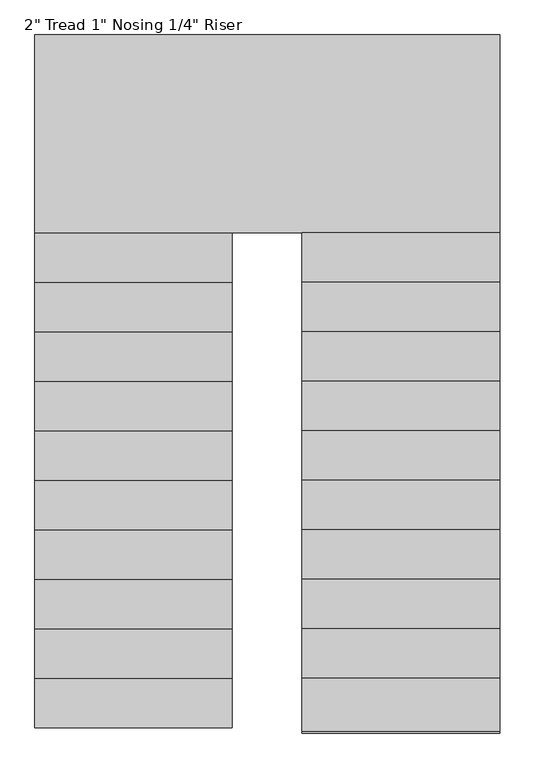
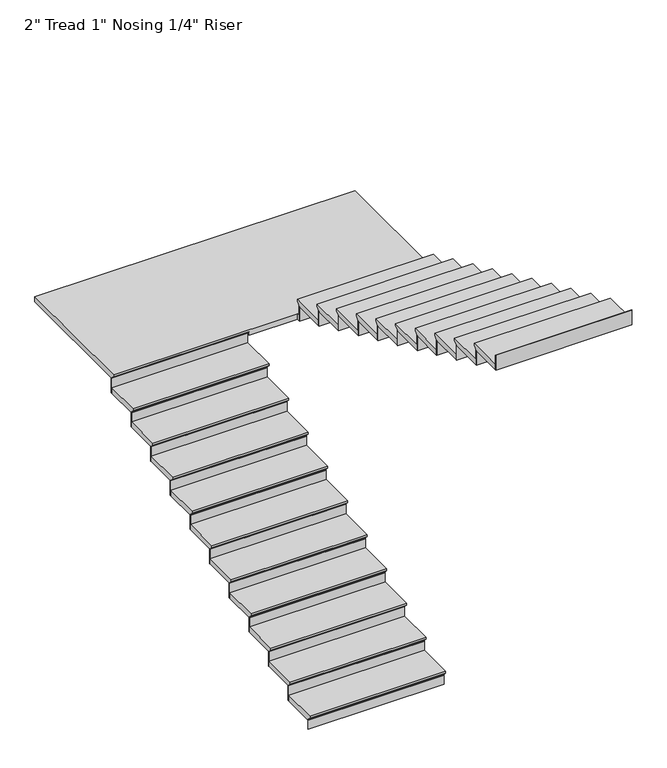
"""IFC4 building model written with IfcOpenShell, lengths in millimetres: stair flight geometry."""

from ifc_helpers import new_model, si_unit, origin, place, context, project, spatial, faceted_brep, source, transform, mapped, element, save


def stair_flight_5ae6432b(model_context):
    return source(origin(), model_context, "Body", "Brep", [
        faceted_brep([(-629.5987998, 3364.6067329, 6520.2954545), (-629.5987998, 3364.6067329, 6539.3454545), (-1845.5417538, 3364.6067329, 6539.3454545), (-1845.5417538, 3364.6067329, 6520.2954545), (-629.5987998, 3390.0067329, 6494.8954545), (-1845.5417538, 3390.0067329, 6494.8954545), (-629.5987998, 3694.8067329, 6539.3454545), (-1845.5417538, 3694.8067329, 6539.3454545), (-1845.5417538, 3390.0067329, 6488.5454545), (-1845.5417538, 3694.8067329, 6488.5454545), (-629.5987998, 3694.8067329, 6488.5454545), (-629.5987998, 3390.0067329, 6488.5454545)], [[[0, 1, 2, 3]], [[4, 0, 3, 5]], [[2, 1, 6, 7]], [[8, 9, 10, 11]], [[2, 7, 9, 8, 5, 3]], [[8, 11, 4, 5]], [[6, 1, 0, 4, 11, 10]], [[7, 6, 10, 9]]]),
        faceted_brep([(-629.5987998, 3390.0067329, 6488.5454545), (-629.5987998, 3390.0067329, 6400.8), (-629.5987998, 3396.3567329, 6400.8), (-629.5987998, 3396.3567329, 6488.5454545), (-1845.5417538, 3390.0067329, 6488.5454545), (-1845.5417538, 3396.3567329, 6488.5454545), (-1845.5417538, 3396.3567329, 6400.8), (-1845.5417538, 3390.0067329, 6400.8)], [[[0, 1, 2, 3]], [[4, 5, 6, 7]], [[1, 0, 4, 7]], [[2, 1, 7, 6]], [[3, 2, 6, 5]], [[0, 3, 5, 4]]]),
        faceted_brep([(-629.5987998, 3694.8067329, 6627.0909091), (-629.5987998, 3694.8067329, 6488.5454545), (-629.5987998, 3701.1567329, 6488.5454545), (-629.5987998, 3701.1567329, 6627.0909091), (-1845.5417538, 3694.8067329, 6627.0909091), (-1845.5417538, 3701.1567329, 6627.0909091), (-1845.5417538, 3701.1567329, 6488.5454545), (-1845.5417538, 3694.8067329, 6488.5454545)], [[[0, 1, 2, 3]], [[4, 5, 6, 7]], [[1, 0, 4, 7]], [[2, 1, 7, 6]], [[3, 2, 6, 5]], [[0, 3, 5, 4]]]),
        faceted_brep([(-1845.5417538, 3669.4067329, 6677.8909091), (-629.5987998, 3669.4067329, 6677.8909091), (-629.5987998, 3999.6067329, 6677.8909091), (-1845.5417538, 3999.6067329, 6677.8909091), (-1845.5417538, 3694.8067329, 6627.0909091), (-1845.5417538, 3999.6067329, 6627.0909091), (-629.5987998, 3999.6067329, 6627.0909091), (-629.5987998, 3694.8067329, 6627.0909091), (-1845.5417538, 3694.8067329, 6633.4409091), (-1845.5417538, 3669.4067329, 6658.8409091), (-629.5987998, 3694.8067329, 6633.4409091), (-629.5987998, 3669.4067329, 6658.8409091)], [[[0, 1, 2, 3]], [[4, 5, 6, 7]], [[0, 3, 5, 4, 8, 9]], [[4, 7, 10, 8]], [[2, 1, 11, 10, 7, 6]], [[3, 2, 6, 5]], [[11, 1, 0, 9]], [[10, 11, 9, 8]]]),
        faceted_brep([(-629.5987998, 3999.6067329, 6765.6363636), (-629.5987998, 3999.6067329, 6627.0909091), (-629.5987998, 4005.9567329, 6627.0909091), (-629.5987998, 4005.9567329, 6765.6363636), (-1845.5417538, 3999.6067329, 6765.6363636), (-1845.5417538, 4005.9567329, 6765.6363636), (-1845.5417538, 4005.9567329, 6627.0909091), (-1845.5417538, 3999.6067329, 6627.0909091)], [[[0, 1, 2, 3]], [[4, 5, 6, 7]], [[1, 0, 4, 7]], [[2, 1, 7, 6]], [[3, 2, 6, 5]], [[0, 3, 5, 4]]]),
        faceted_brep([(-1845.5417538, 3974.2067329, 6816.4363636), (-629.5987998, 3974.2067329, 6816.4363636), (-629.5987998, 4304.4067329, 6816.4363636), (-1845.5417538, 4304.4067329, 6816.4363636), (-1845.5417538, 3999.6067329, 6765.6363636), (-1845.5417538, 4304.4067329, 6765.6363636), (-629.5987998, 4304.4067329, 6765.6363636), (-629.5987998, 3999.6067329, 6765.6363636), (-1845.5417538, 3999.6067329, 6771.9863636), (-1845.5417538, 3974.2067329, 6797.3863636), (-629.5987998, 3999.6067329, 6771.9863636), (-629.5987998, 3974.2067329, 6797.3863636)], [[[0, 1, 2, 3]], [[4, 5, 6, 7]], [[0, 3, 5, 4, 8, 9]], [[4, 7, 10, 8]], [[2, 1, 11, 10, 7, 6]], [[3, 2, 6, 5]], [[11, 1, 0, 9]], [[10, 11, 9, 8]]]),
        faceted_brep([(-629.5987998, 4304.4067329, 6904.1818182), (-629.5987998, 4304.4067329, 6765.6363636), (-629.5987998, 4310.7567329, 6765.6363636), (-629.5987998, 4310.7567329, 6904.1818182), (-1845.5417538, 4304.4067329, 6904.1818182), (-1845.5417538, 4310.7567329, 6904.1818182), (-1845.5417538, 4310.7567329, 6765.6363636), (-1845.5417538, 4304.4067329, 6765.6363636)], [[[0, 1, 2, 3]], [[4, 5, 6, 7]], [[1, 0, 4, 7]], [[2, 1, 7, 6]], [[3, 2, 6, 5]], [[0, 3, 5, 4]]]),
        faceted_brep([(-1845.5417538, 4279.0067329, 6954.9818182), (-629.5987998, 4279.0067329, 6954.9818182), (-629.5987998, 4609.2067329, 6954.9818182), (-1845.5417538, 4609.2067329, 6954.9818182), (-1845.5417538, 4304.4067329, 6904.1818182), (-1845.5417538, 4609.2067329, 6904.1818182), (-629.5987998, 4609.2067329, 6904.1818182), (-629.5987998, 4304.4067329, 6904.1818182), (-1845.5417538, 4304.4067329, 6910.5318182), (-1845.5417538, 4279.0067329, 6935.9318182), (-629.5987998, 4304.4067329, 6910.5318182), (-629.5987998, 4279.0067329, 6935.9318182)], [[[0, 1, 2, 3]], [[4, 5, 6, 7]], [[0, 3, 5, 4, 8, 9]], [[4, 7, 10, 8]], [[2, 1, 11, 10, 7, 6]], [[3, 2, 6, 5]], [[11, 1, 0, 9]], [[10, 11, 9, 8]]]),
        faceted_brep([(-629.5987998, 4609.2067329, 7042.7272727), (-629.5987998, 4609.2067329, 6904.1818182), (-629.5987998, 4615.5567329, 6904.1818182), (-629.5987998, 4615.5567329, 7042.7272727), (-1845.5417538, 4609.2067329, 7042.7272727), (-1845.5417538, 4615.5567329, 7042.7272727), (-1845.5417538, 4615.5567329, 6904.1818182), (-1845.5417538, 4609.2067329, 6904.1818182)], [[[0, 1, 2, 3]], [[4, 5, 6, 7]], [[1, 0, 4, 7]], [[2, 1, 7, 6]], [[3, 2, 6, 5]], [[0, 3, 5, 4]]]),
        faceted_brep([(-1845.5417538, 4583.8067329, 7093.5272727), (-629.5987998, 4583.8067329, 7093.5272727), (-629.5987998, 4914.0067329, 7093.5272727), (-1845.5417538, 4914.0067329, 7093.5272727), (-1845.5417538, 4609.2067329, 7042.7272727), (-1845.5417538, 4914.0067329, 7042.7272727), (-629.5987998, 4914.0067329, 7042.7272727), (-629.5987998, 4609.2067329, 7042.7272727), (-1845.5417538, 4609.2067329, 7049.0772727), (-1845.5417538, 4583.8067329, 7074.4772727), (-629.5987998, 4609.2067329, 7049.0772727), (-629.5987998, 4583.8067329, 7074.4772727)], [[[0, 1, 2, 3]], [[4, 5, 6, 7]], [[0, 3, 5, 4, 8, 9]], [[4, 7, 10, 8]], [[2, 1, 11, 10, 7, 6]], [[3, 2, 6, 5]], [[11, 1, 0, 9]], [[10, 11, 9, 8]]]),
        faceted_brep([(-629.5987998, 4914.0067329, 7181.2727273), (-629.5987998, 4914.0067329, 7042.7272727), (-629.5987998, 4920.3567329, 7042.7272727), (-629.5987998, 4920.3567329, 7181.2727273), (-1845.5417538, 4914.0067329, 7181.2727273), (-1845.5417538, 4920.3567329, 7181.2727273), (-1845.5417538, 4920.3567329, 7042.7272727), (-1845.5417538, 4914.0067329, 7042.7272727)], [[[0, 1, 2, 3]], [[4, 5, 6, 7]], [[1, 0, 4, 7]], [[2, 1, 7, 6]], [[3, 2, 6, 5]], [[0, 3, 5, 4]]]),
        faceted_brep([(-1845.5417538, 4888.6067329, 7232.0727273), (-629.5987998, 4888.6067329, 7232.0727273), (-629.5987998, 5218.8067329, 7232.0727273), (-1845.5417538, 5218.8067329, 7232.0727273), (-1845.5417538, 4914.0067329, 7181.2727273), (-1845.5417538, 5218.8067329, 7181.2727273), (-629.5987998, 5218.8067329, 7181.2727273), (-629.5987998, 4914.0067329, 7181.2727273), (-1845.5417538, 4914.0067329, 7187.6227273), (-1845.5417538, 4888.6067329, 7213.0227273), (-629.5987998, 4914.0067329, 7187.6227273), (-629.5987998, 4888.6067329, 7213.0227273)], [[[0, 1, 2, 3]], [[4, 5, 6, 7]], [[0, 3, 5, 4, 8, 9]], [[4, 7, 10, 8]], [[2, 1, 11, 10, 7, 6]], [[3, 2, 6, 5]], [[11, 1, 0, 9]], [[10, 11, 9, 8]]]),
        faceted_brep([(-629.5987998, 5218.8067329, 7319.8181818), (-629.5987998, 5218.8067329, 7181.2727273), (-629.5987998, 5225.1567329, 7181.2727273), (-629.5987998, 5225.1567329, 7319.8181818), (-1845.5417538, 5218.8067329, 7319.8181818), (-1845.5417538, 5225.1567329, 7319.8181818), (-1845.5417538, 5225.1567329, 7181.2727273), (-1845.5417538, 5218.8067329, 7181.2727273)], [[[0, 1, 2, 3]], [[4, 5, 6, 7]], [[1, 0, 4, 7]], [[2, 1, 7, 6]], [[3, 2, 6, 5]], [[0, 3, 5, 4]]]),
        faceted_brep([(-1845.5417538, 5193.4067329, 7370.6181818), (-629.5987998, 5193.4067329, 7370.6181818), (-629.5987998, 5523.6067329, 7370.6181818), (-1845.5417538, 5523.6067329, 7370.6181818), (-1845.5417538, 5218.8067329, 7319.8181818), (-1845.5417538, 5523.6067329, 7319.8181818), (-629.5987998, 5523.6067329, 7319.8181818), (-629.5987998, 5218.8067329, 7319.8181818), (-1845.5417538, 5218.8067329, 7326.1681818), (-1845.5417538, 5193.4067329, 7351.5681818), (-629.5987998, 5218.8067329, 7326.1681818), (-629.5987998, 5193.4067329, 7351.5681818)], [[[0, 1, 2, 3]], [[4, 5, 6, 7]], [[0, 3, 5, 4, 8, 9]], [[4, 7, 10, 8]], [[2, 1, 11, 10, 7, 6]], [[3, 2, 6, 5]], [[11, 1, 0, 9]], [[10, 11, 9, 8]]]),
        faceted_brep([(-629.5987998, 5523.6067329, 7458.3636364), (-629.5987998, 5523.6067329, 7319.8181818), (-629.5987998, 5529.9567329, 7319.8181818), (-629.5987998, 5529.9567329, 7458.3636364), (-1845.5417538, 5523.6067329, 7458.3636364), (-1845.5417538, 5529.9567329, 7458.3636364), (-1845.5417538, 5529.9567329, 7319.8181818), (-1845.5417538, 5523.6067329, 7319.8181818)], [[[0, 1, 2, 3]], [[4, 5, 6, 7]], [[1, 0, 4, 7]], [[2, 1, 7, 6]], [[3, 2, 6, 5]], [[0, 3, 5, 4]]]),
        faceted_brep([(-1845.5417538, 5498.2067329, 7509.1636364), (-629.5987998, 5498.2067329, 7509.1636364), (-629.5987998, 5828.4067329, 7509.1636364), (-1845.5417538, 5828.4067329, 7509.1636364), (-1845.5417538, 5523.6067329, 7458.3636364), (-1845.5417538, 5828.4067329, 7458.3636364), (-629.5987998, 5828.4067329, 7458.3636364), (-629.5987998, 5523.6067329, 7458.3636364), (-1845.5417538, 5523.6067329, 7464.7136364), (-1845.5417538, 5498.2067329, 7490.1136364), (-629.5987998, 5523.6067329, 7464.7136364), (-629.5987998, 5498.2067329, 7490.1136364)], [[[0, 1, 2, 3]], [[4, 5, 6, 7]], [[0, 3, 5, 4, 8, 9]], [[4, 7, 10, 8]], [[2, 1, 11, 10, 7, 6]], [[3, 2, 6, 5]], [[11, 1, 0, 9]], [[10, 11, 9, 8]]]),
        faceted_brep([(-629.5987998, 5828.4067329, 7596.9090909), (-629.5987998, 5828.4067329, 7458.3636364), (-629.5987998, 5834.7567329, 7458.3636364), (-629.5987998, 5834.7567329, 7596.9090909), (-1845.5417538, 5828.4067329, 7596.9090909), (-1845.5417538, 5834.7567329, 7596.9090909), (-1845.5417538, 5834.7567329, 7458.3636364), (-1845.5417538, 5828.4067329, 7458.3636364)], [[[0, 1, 2, 3]], [[4, 5, 6, 7]], [[1, 0, 4, 7]], [[2, 1, 7, 6]], [[3, 2, 6, 5]], [[0, 3, 5, 4]]]),
        faceted_brep([(-1845.5417538, 5803.0067329, 7647.7090909), (-629.5987998, 5803.0067329, 7647.7090909), (-629.5987998, 6133.2067329, 7647.7090909), (-1845.5417538, 6133.2067329, 7647.7090909), (-1845.5417538, 5828.4067329, 7596.9090909), (-1845.5417538, 6133.2067329, 7596.9090909), (-629.5987998, 6133.2067329, 7596.9090909), (-629.5987998, 5828.4067329, 7596.9090909), (-1845.5417538, 5828.4067329, 7603.2590909), (-1845.5417538, 5803.0067329, 7628.6590909), (-629.5987998, 5828.4067329, 7603.2590909), (-629.5987998, 5803.0067329, 7628.6590909)], [[[0, 1, 2, 3]], [[4, 5, 6, 7]], [[0, 3, 5, 4, 8, 9]], [[4, 7, 10, 8]], [[2, 1, 11, 10, 7, 6]], [[3, 2, 6, 5]], [[11, 1, 0, 9]], [[10, 11, 9, 8]]]),
        faceted_brep([(-629.5987998, 6133.2067329, 7735.4545455), (-629.5987998, 6133.2067329, 7596.9090909), (-629.5987998, 6139.5567329, 7596.9090909), (-629.5987998, 6139.5567329, 7735.4545455), (-1845.5417538, 6133.2067329, 7735.4545455), (-1845.5417538, 6139.5567329, 7735.4545455), (-1845.5417538, 6139.5567329, 7596.9090909), (-1845.5417538, 6133.2067329, 7596.9090909)], [[[0, 1, 2, 3]], [[4, 5, 6, 7]], [[1, 0, 4, 7]], [[2, 1, 7, 6]], [[3, 2, 6, 5]], [[0, 3, 5, 4]]]),
        faceted_brep([(-1845.5417538, 6107.8067329, 7786.2545455), (-629.5987998, 6107.8067329, 7786.2545455), (-629.5987998, 6438.0067329, 7786.2545455), (-1845.5417538, 6438.0067329, 7786.2545455), (-1845.5417538, 6133.2067329, 7735.4545455), (-1845.5417538, 6438.0067329, 7735.4545455), (-629.5987998, 6438.0067329, 7735.4545455), (-629.5987998, 6133.2067329, 7735.4545455), (-1845.5417538, 6133.2067329, 7741.8045455), (-1845.5417538, 6107.8067329, 7767.2045455), (-629.5987998, 6133.2067329, 7741.8045455), (-629.5987998, 6107.8067329, 7767.2045455)], [[[0, 1, 2, 3]], [[4, 5, 6, 7]], [[0, 3, 5, 4, 8, 9]], [[4, 7, 10, 8]], [[2, 1, 11, 10, 7, 6]], [[3, 2, 6, 5]], [[11, 1, 0, 9]], [[10, 11, 9, 8]]]),
        faceted_brep([(-629.5987998, 6438.0067329, 7874.0), (-629.5987998, 6438.0067329, 7735.4545455), (-629.5987998, 6444.3567329, 7735.4545455), (-629.5987998, 6444.3567329, 7874.0), (-1845.5417538, 6438.0067329, 7874.0), (-1845.5417538, 6444.3567329, 7874.0), (-1845.5417538, 6444.3567329, 7735.4545455), (-1845.5417538, 6438.0067329, 7735.4545455)], [[[0, 1, 2, 3]], [[4, 5, 6, 7]], [[1, 0, 4, 7]], [[2, 1, 7, 6]], [[3, 2, 6, 5]], [[0, 3, 5, 4]]]),
        faceted_brep([(1021.4012085, 6387.2067329, 7924.8), (1021.4012085, 7631.8067329, 7924.8), (-1845.5417538, 7631.8067329, 7924.8), (-1845.5417538, 6412.6067329, 7924.8), (-197.7987915, 6412.6067329, 7924.8), (-197.7987915, 6387.2067329, 7924.8), (1021.4012085, 7631.8067329, 7874.0), (1021.4012085, 6387.2067329, 7874.0), (-197.7987915, 6387.2067329, 7874.0), (-197.7987915, 6412.6067329, 7874.0), (-629.5987998, 6412.6067329, 7874.0), (-629.5987998, 6438.0067329, 7874.0), (-1845.5417538, 6438.0067329, 7874.0), (-1845.5417538, 7631.8067329, 7874.0), (-629.5987998, 6438.0067329, 7880.35), (-1845.5417538, 6438.0067329, 7880.35), (-1845.5417538, 6412.6067329, 7905.75), (-629.5987998, 6412.6067329, 7905.75)], [[[0, 1, 2, 3, 4, 5]], [[6, 7, 8, 9, 10, 11, 12, 13]], [[1, 0, 7, 6]], [[2, 1, 6, 13]], [[12, 11, 14, 15]], [[4, 3, 16, 17, 10, 9]], [[5, 4, 9, 8]], [[0, 5, 8, 7]], [[16, 15, 14, 17]], [[3, 2, 13, 12, 15, 16]], [[11, 10, 17, 14]]]),
        faceted_brep([(-197.7987915, 6387.2067329, 8012.5454545), (-197.7987915, 6387.2067329, 7874.0), (-197.7987915, 6380.8567329, 7874.0), (-197.7987915, 6380.8567329, 8012.5454545), (1021.4012085, 6387.2067329, 8012.5454545), (1021.4012085, 6380.8567329, 8012.5454545), (1021.4012085, 6380.8567329, 7874.0), (1021.4012085, 6387.2067329, 7874.0)], [[[0, 1, 2, 3]], [[4, 5, 6, 7]], [[1, 0, 4, 7]], [[2, 1, 7, 6]], [[3, 2, 6, 5]], [[0, 3, 5, 4]]]),
        faceted_brep([(1021.4012085, 6412.6067329, 8063.3454545), (-197.7987915, 6412.6067329, 8063.3454545), (-197.7987915, 6082.4067329, 8063.3454545), (1021.4012085, 6082.4067329, 8063.3454545), (1021.4012085, 6387.2067329, 8012.5454545), (1021.4012085, 6082.4067329, 8012.5454545), (-197.7987915, 6082.4067329, 8012.5454545), (-197.7987915, 6387.2067329, 8012.5454545), (1021.4012085, 6387.2067329, 8018.8954545), (1021.4012085, 6412.6067329, 8044.2954545), (-197.7987915, 6387.2067329, 8018.8954545), (-197.7987915, 6412.6067329, 8044.2954545)], [[[0, 1, 2, 3]], [[4, 5, 6, 7]], [[0, 3, 5, 4, 8, 9]], [[4, 7, 10, 8]], [[2, 1, 11, 10, 7, 6]], [[3, 2, 6, 5]], [[11, 1, 0, 9]], [[10, 11, 9, 8]]]),
        faceted_brep([(-197.7987915, 6082.4067329, 8151.0909091), (-197.7987915, 6082.4067329, 8012.5454545), (-197.7987915, 6076.0567329, 8012.5454545), (-197.7987915, 6076.0567329, 8151.0909091), (1021.4012085, 6082.4067329, 8151.0909091), (1021.4012085, 6076.0567329, 8151.0909091), (1021.4012085, 6076.0567329, 8012.5454545), (1021.4012085, 6082.4067329, 8012.5454545)], [[[0, 1, 2, 3]], [[4, 5, 6, 7]], [[1, 0, 4, 7]], [[2, 1, 7, 6]], [[3, 2, 6, 5]], [[0, 3, 5, 4]]]),
        faceted_brep([(1021.4012085, 6107.8067329, 8201.8909091), (-197.7987915, 6107.8067329, 8201.8909091), (-197.7987915, 5777.6067329, 8201.8909091), (1021.4012085, 5777.6067329, 8201.8909091), (1021.4012085, 6082.4067329, 8151.0909091), (1021.4012085, 5777.6067329, 8151.0909091), (-197.7987915, 5777.6067329, 8151.0909091), (-197.7987915, 6082.4067329, 8151.0909091), (1021.4012085, 6082.4067329, 8157.4409091), (1021.4012085, 6107.8067329, 8182.8409091), (-197.7987915, 6082.4067329, 8157.4409091), (-197.7987915, 6107.8067329, 8182.8409091)], [[[0, 1, 2, 3]], [[4, 5, 6, 7]], [[0, 3, 5, 4, 8, 9]], [[4, 7, 10, 8]], [[2, 1, 11, 10, 7, 6]], [[3, 2, 6, 5]], [[11, 1, 0, 9]], [[10, 11, 9, 8]]]),
        faceted_brep([(-197.7987915, 5777.6067329, 8289.6363636), (-197.7987915, 5777.6067329, 8151.0909091), (-197.7987915, 5771.2567329, 8151.0909091), (-197.7987915, 5771.2567329, 8289.6363636), (1021.4012085, 5777.6067329, 8289.6363636), (1021.4012085, 5771.2567329, 8289.6363636), (1021.4012085, 5771.2567329, 8151.0909091), (1021.4012085, 5777.6067329, 8151.0909091)], [[[0, 1, 2, 3]], [[4, 5, 6, 7]], [[1, 0, 4, 7]], [[2, 1, 7, 6]], [[3, 2, 6, 5]], [[0, 3, 5, 4]]]),
        faceted_brep([(1021.4012085, 5803.0067329, 8340.4363636), (-197.7987915, 5803.0067329, 8340.4363636), (-197.7987915, 5472.8067329, 8340.4363636), (1021.4012085, 5472.8067329, 8340.4363636), (1021.4012085, 5777.6067329, 8289.6363636), (1021.4012085, 5472.8067329, 8289.6363636), (-197.7987915, 5472.8067329, 8289.6363636), (-197.7987915, 5777.6067329, 8289.6363636), (1021.4012085, 5777.6067329, 8295.9863636), (1021.4012085, 5803.0067329, 8321.3863636), (-197.7987915, 5777.6067329, 8295.9863636), (-197.7987915, 5803.0067329, 8321.3863636)], [[[0, 1, 2, 3]], [[4, 5, 6, 7]], [[0, 3, 5, 4, 8, 9]], [[4, 7, 10, 8]], [[2, 1, 11, 10, 7, 6]], [[3, 2, 6, 5]], [[11, 1, 0, 9]], [[10, 11, 9, 8]]]),
        faceted_brep([(-197.7987915, 5472.8067329, 8428.1818182), (-197.7987915, 5472.8067329, 8289.6363636), (-197.7987915, 5466.4567329, 8289.6363636), (-197.7987915, 5466.4567329, 8428.1818182), (1021.4012085, 5472.8067329, 8428.1818182), (1021.4012085, 5466.4567329, 8428.1818182), (1021.4012085, 5466.4567329, 8289.6363636), (1021.4012085, 5472.8067329, 8289.6363636)], [[[0, 1, 2, 3]], [[4, 5, 6, 7]], [[1, 0, 4, 7]], [[2, 1, 7, 6]], [[3, 2, 6, 5]], [[0, 3, 5, 4]]]),
        faceted_brep([(1021.4012085, 5498.2067329, 8478.9818182), (-197.7987915, 5498.2067329, 8478.9818182), (-197.7987915, 5168.0067329, 8478.9818182), (1021.4012085, 5168.0067329, 8478.9818182), (1021.4012085, 5472.8067329, 8428.1818182), (1021.4012085, 5168.0067329, 8428.1818182), (-197.7987915, 5168.0067329, 8428.1818182), (-197.7987915, 5472.8067329, 8428.1818182), (1021.4012085, 5472.8067329, 8434.5318182), (1021.4012085, 5498.2067329, 8459.9318182), (-197.7987915, 5472.8067329, 8434.5318182), (-197.7987915, 5498.2067329, 8459.9318182)], [[[0, 1, 2, 3]], [[4, 5, 6, 7]], [[0, 3, 5, 4, 8, 9]], [[4, 7, 10, 8]], [[2, 1, 11, 10, 7, 6]], [[3, 2, 6, 5]], [[11, 1, 0, 9]], [[10, 11, 9, 8]]]),
        faceted_brep([(-197.7987915, 5168.0067329, 8566.7272727), (-197.7987915, 5168.0067329, 8428.1818182), (-197.7987915, 5161.6567329, 8428.1818182), (-197.7987915, 5161.6567329, 8566.7272727), (1021.4012085, 5168.0067329, 8566.7272727), (1021.4012085, 5161.6567329, 8566.7272727), (1021.4012085, 5161.6567329, 8428.1818182), (1021.4012085, 5168.0067329, 8428.1818182)], [[[0, 1, 2, 3]], [[4, 5, 6, 7]], [[1, 0, 4, 7]], [[2, 1, 7, 6]], [[3, 2, 6, 5]], [[0, 3, 5, 4]]]),
        faceted_brep([(1021.4012085, 5193.4067329, 8617.5272727), (-197.7987915, 5193.4067329, 8617.5272727), (-197.7987915, 4863.2067329, 8617.5272727), (1021.4012085, 4863.2067329, 8617.5272727), (1021.4012085, 5168.0067329, 8566.7272727), (1021.4012085, 4863.2067329, 8566.7272727), (-197.7987915, 4863.2067329, 8566.7272727), (-197.7987915, 5168.0067329, 8566.7272727), (1021.4012085, 5168.0067329, 8573.0772727), (1021.4012085, 5193.4067329, 8598.4772727), (-197.7987915, 5168.0067329, 8573.0772727), (-197.7987915, 5193.4067329, 8598.4772727)], [[[0, 1, 2, 3]], [[4, 5, 6, 7]], [[0, 3, 5, 4, 8, 9]], [[4, 7, 10, 8]], [[2, 1, 11, 10, 7, 6]], [[3, 2, 6, 5]], [[11, 1, 0, 9]], [[10, 11, 9, 8]]]),
        faceted_brep([(-197.7987915, 4863.2067329, 8705.2727273), (-197.7987915, 4863.2067329, 8566.7272727), (-197.7987915, 4856.8567329, 8566.7272727), (-197.7987915, 4856.8567329, 8705.2727273), (1021.4012085, 4863.2067329, 8705.2727273), (1021.4012085, 4856.8567329, 8705.2727273), (1021.4012085, 4856.8567329, 8566.7272727), (1021.4012085, 4863.2067329, 8566.7272727)], [[[0, 1, 2, 3]], [[4, 5, 6, 7]], [[1, 0, 4, 7]], [[2, 1, 7, 6]], [[3, 2, 6, 5]], [[0, 3, 5, 4]]]),
        faceted_brep([(1021.4012085, 4888.6067329, 8756.0727273), (-197.7987915, 4888.6067329, 8756.0727273), (-197.7987915, 4558.4067329, 8756.0727273), (1021.4012085, 4558.4067329, 8756.0727273), (1021.4012085, 4863.2067329, 8705.2727273), (1021.4012085, 4558.4067329, 8705.2727273), (-197.7987915, 4558.4067329, 8705.2727273), (-197.7987915, 4863.2067329, 8705.2727273), (1021.4012085, 4863.2067329, 8711.6227273), (1021.4012085, 4888.6067329, 8737.0227273), (-197.7987915, 4863.2067329, 8711.6227273), (-197.7987915, 4888.6067329, 8737.0227273)], [[[0, 1, 2, 3]], [[4, 5, 6, 7]], [[0, 3, 5, 4, 8, 9]], [[4, 7, 10, 8]], [[2, 1, 11, 10, 7, 6]], [[3, 2, 6, 5]], [[11, 1, 0, 9]], [[10, 11, 9, 8]]]),
        faceted_brep([(-197.7987915, 4558.4067329, 8843.8181818), (-197.7987915, 4558.4067329, 8705.2727273), (-197.7987915, 4552.0567329, 8705.2727273), (-197.7987915, 4552.0567329, 8843.8181818), (1021.4012085, 4558.4067329, 8843.8181818), (1021.4012085, 4552.0567329, 8843.8181818), (1021.4012085, 4552.0567329, 8705.2727273), (1021.4012085, 4558.4067329, 8705.2727273)], [[[0, 1, 2, 3]], [[4, 5, 6, 7]], [[1, 0, 4, 7]], [[2, 1, 7, 6]], [[3, 2, 6, 5]], [[0, 3, 5, 4]]]),
        faceted_brep([(1021.4012085, 4583.8067329, 8894.6181818), (-197.7987915, 4583.8067329, 8894.6181818), (-197.7987915, 4253.6067329, 8894.6181818), (1021.4012085, 4253.6067329, 8894.6181818), (1021.4012085, 4558.4067329, 8843.8181818), (1021.4012085, 4253.6067329, 8843.8181818), (-197.7987915, 4253.6067329, 8843.8181818), (-197.7987915, 4558.4067329, 8843.8181818), (1021.4012085, 4558.4067329, 8850.1681818), (1021.4012085, 4583.8067329, 8875.5681818), (-197.7987915, 4558.4067329, 8850.1681818), (-197.7987915, 4583.8067329, 8875.5681818)], [[[0, 1, 2, 3]], [[4, 5, 6, 7]], [[0, 3, 5, 4, 8, 9]], [[4, 7, 10, 8]], [[2, 1, 11, 10, 7, 6]], [[3, 2, 6, 5]], [[11, 1, 0, 9]], [[10, 11, 9, 8]]]),
        faceted_brep([(-197.7987915, 4253.6067329, 8982.3636364), (-197.7987915, 4253.6067329, 8843.8181818), (-197.7987915, 4247.2567329, 8843.8181818), (-197.7987915, 4247.2567329, 8982.3636364), (1021.4012085, 4253.6067329, 8982.3636364), (1021.4012085, 4247.2567329, 8982.3636364), (1021.4012085, 4247.2567329, 8843.8181818), (1021.4012085, 4253.6067329, 8843.8181818)], [[[0, 1, 2, 3]], [[4, 5, 6, 7]], [[1, 0, 4, 7]], [[2, 1, 7, 6]], [[3, 2, 6, 5]], [[0, 3, 5, 4]]]),
        faceted_brep([(1021.4012085, 4279.0067329, 9033.1636364), (-197.7987915, 4279.0067329, 9033.1636364), (-197.7987915, 3948.8067329, 9033.1636364), (1021.4012085, 3948.8067329, 9033.1636364), (1021.4012085, 4253.6067329, 8982.3636364), (1021.4012085, 3948.8067329, 8982.3636364), (-197.7987915, 3948.8067329, 8982.3636364), (-197.7987915, 4253.6067329, 8982.3636364), (1021.4012085, 4253.6067329, 8988.7136364), (1021.4012085, 4279.0067329, 9014.1136364), (-197.7987915, 4253.6067329, 8988.7136364), (-197.7987915, 4279.0067329, 9014.1136364)], [[[0, 1, 2, 3]], [[4, 5, 6, 7]], [[0, 3, 5, 4, 8, 9]], [[4, 7, 10, 8]], [[2, 1, 11, 10, 7, 6]], [[3, 2, 6, 5]], [[11, 1, 0, 9]], [[10, 11, 9, 8]]]),
        faceted_brep([(-197.7987915, 3948.8067329, 9120.9090909), (-197.7987915, 3948.8067329, 8982.3636364), (-197.7987915, 3942.4567329, 8982.3636364), (-197.7987915, 3942.4567329, 9120.9090909), (1021.4012085, 3948.8067329, 9120.9090909), (1021.4012085, 3942.4567329, 9120.9090909), (1021.4012085, 3942.4567329, 8982.3636364), (1021.4012085, 3948.8067329, 8982.3636364)], [[[0, 1, 2, 3]], [[4, 5, 6, 7]], [[1, 0, 4, 7]], [[2, 1, 7, 6]], [[3, 2, 6, 5]], [[0, 3, 5, 4]]]),
        faceted_brep([(1021.4012085, 3974.2067329, 9171.7090909), (-197.7987915, 3974.2067329, 9171.7090909), (-197.7987915, 3644.0067329, 9171.7090909), (1021.4012085, 3644.0067329, 9171.7090909), (1021.4012085, 3948.8067329, 9120.9090909), (1021.4012085, 3644.0067329, 9120.9090909), (-197.7987915, 3644.0067329, 9120.9090909), (-197.7987915, 3948.8067329, 9120.9090909), (1021.4012085, 3948.8067329, 9127.2590909), (1021.4012085, 3974.2067329, 9152.6590909), (-197.7987915, 3948.8067329, 9127.2590909), (-197.7987915, 3974.2067329, 9152.6590909)], [[[0, 1, 2, 3]], [[4, 5, 6, 7]], [[0, 3, 5, 4, 8, 9]], [[4, 7, 10, 8]], [[2, 1, 11, 10, 7, 6]], [[3, 2, 6, 5]], [[11, 1, 0, 9]], [[10, 11, 9, 8]]]),
        faceted_brep([(-197.7987915, 3644.0067329, 9259.4545455), (-197.7987915, 3644.0067329, 9120.9090909), (-197.7987915, 3637.6567329, 9120.9090909), (-197.7987915, 3637.6567329, 9259.4545455), (1021.4012085, 3644.0067329, 9259.4545455), (1021.4012085, 3637.6567329, 9259.4545455), (1021.4012085, 3637.6567329, 9120.9090909), (1021.4012085, 3644.0067329, 9120.9090909)], [[[0, 1, 2, 3]], [[4, 5, 6, 7]], [[1, 0, 4, 7]], [[2, 1, 7, 6]], [[3, 2, 6, 5]], [[0, 3, 5, 4]]]),
        faceted_brep([(-197.7987915, 3339.2067329, 9398.0), (-197.7987915, 3339.2067329, 9259.4545455), (-197.7987915, 3332.8567329, 9259.4545455), (-197.7987915, 3332.8567329, 9398.0), (1021.4012085, 3339.2067329, 9398.0), (1021.4012085, 3332.8567329, 9398.0), (1021.4012085, 3332.8567329, 9259.4545455), (1021.4012085, 3339.2067329, 9259.4545455)], [[[0, 1, 2, 3]], [[4, 5, 6, 7]], [[1, 0, 4, 7]], [[2, 1, 7, 6]], [[3, 2, 6, 5]], [[0, 3, 5, 4]]]),
        faceted_brep([(1021.4012085, 3669.4067329, 9310.2545455), (-197.7987915, 3669.4067329, 9310.2545455), (-197.7987915, 3339.2067329, 9310.2545455), (1021.4012085, 3339.2067329, 9310.2545455), (1021.4012085, 3644.0067329, 9259.4545455), (1021.4012085, 3339.2067329, 9259.4545455), (-197.7987915, 3339.2067329, 9259.4545455), (-197.7987915, 3644.0067329, 9259.4545455), (1021.4012085, 3644.0067329, 9265.8045455), (1021.4012085, 3669.4067329, 9291.2045455), (-197.7987915, 3644.0067329, 9265.8045455), (-197.7987915, 3669.4067329, 9291.2045455)], [[[0, 1, 2, 3]], [[4, 5, 6, 7]], [[0, 3, 5, 4, 8, 9]], [[4, 7, 10, 8]], [[2, 1, 11, 10, 7, 6]], [[3, 2, 6, 5]], [[11, 1, 0, 9]], [[10, 11, 9, 8]]]),
    ])


if __name__ == "__main__":
    model = new_model("IFC4")
    model_context = context("Model", 3, world=origin())
    ifc_project = project(units=[si_unit("LENGTHUNIT", "METRE", prefix="MILLI")], contexts=[model_context])
    site = spatial("IfcSite", under=ifc_project)
    building = spatial("IfcBuilding", under=site)
    placement = place(None, origin())
    stair_flight_shape = stair_flight_5ae6432b(model_context)
    element("IfcStairFlight", 1, ObjectType="2\" Tread 1\" Nosing 1/4\" Riser", at=placement, inside=building, context=model_context, shape_type="MappedRepresentation", body=[
        mapped(stair_flight_shape, transform((0.0, 0.0, 0.0), x_axis=(1.0, 0.0, 0.0), y_axis=(0.0, 1.0, 0.0), z_axis=(0.0, 0.0, 1.0))),
    ])
    save(model, "model.ifc")
